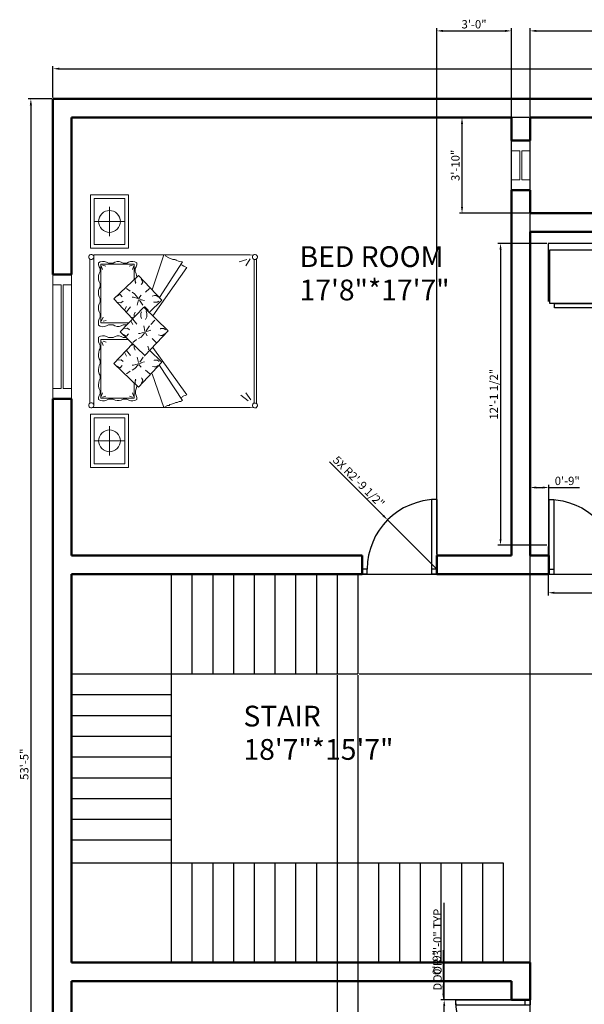
# Model space of a CAD drawing. Units: inches. Extents: x 2201 to 2875, y 1361 to 2074.
# Tile 2 of 4: x 2201 to 2474, y 1600 to 2074. Entities that reach past the tile are written whole.
import ezdxf

# ---------------------------------------------------------------- set-up
doc = ezdxf.new("R2010")
doc.units = ezdxf.units.IN
for name, color, linetype, lineweight in [('A-ANNO-DIMS', 2, 'Continuous', 18), ('A-AREA-IDEN', 7, 'Continuous', 25), ('A-FLOR-FIXT', 9, 'Continuous', 18), ('doors', 5, 'Continuous', 25), ('furniture', 8, 'Continuous', 18), ('stairs', 1, 'Continuous', 25), ('ventilator', 3, 'Continuous', 18), ('walls', 6, 'Continuous', 50), ('windows', 4, 'Continuous', 18)]:
    doc.layers.add(name, color=color, linetype=linetype, lineweight=lineweight)
doc.layers.add('TEFRIŞ', color=11, linetype='Continuous')
doc.styles.get("Standard").update_dxf_attribs({"font": 'arial.ttf'})
doc.dimstyles.new('ISO-25', dxfattribs={"dimtxt": 4, "dimasz": 3, "dimexe": 1.25, "dimexo": 0.625, "dimtad": 1, "dimlunit": 3, "dimtxsty": 'Standard', "dimcen": 2.5, "dimadec": 0, "dimazin": 0, "dimtfac": 1, "dimtmove": 0, "dimatfit": 3, "dimfxl": 1, "dimarcsym": 0})

# ---------------------------------------------------------------- blocks, each defined once
blk = doc.blocks.new('d-bed-3')
at = {"color": 0, "linetype": 'ByBlock'}
for p, q in [((0, 0), (0, -0.5)), ((0.7, 0), (0, 0)), ((0.7, -0.5), (0.7, 0)), ((0.782, -0.005), (0.786, 0.008)), ((0.782, -0.005), (0.786, 0.008)), ((0.786, 0.008), (0.797, 0.017)), ((0.786, 0.008), (0.797, 0.017)), ((0.797, 0.017), (0.808, 0.021)), ((0.797, 0.017), (0.808, 0.021)), ((0.808, 0.021), (0.821, 0.021)), ((0.808, 0.021), (0.821, 0.021)), ((0.821, 0.021), (0.835, 0.014)), ((0.821, 0.021), (0.835, 0.014)), ((0.835, 0.014), (0.841, 0.008)), ((0.835, 0.014), (0.843, 0.006)), ((0.839, 0.008), (2.73, 0.008)), ((0.841, 0.008), (2.73, 0.008)), ((0.843, 0.006), (0.848, -0.008)), ((2.723, -0.008), (2.728, 0.006)), ((2.728, 0.006), (2.736, 0.014)), ((2.73, 0.008), (2.736, 0.014)), ((2.736, 0.014), (2.751, 0.021)), ((2.736, 0.014), (2.751, 0.021)), ((2.751, 0.021), (2.764, 0.021)), ((2.751, 0.021), (2.764, 0.021)), ((2.764, 0.021), (2.775, 0.017)), ((2.764, 0.021), (2.775, 0.017)), ((2.775, 0.017), (2.786, 0.008)), ((2.775, 0.017), (2.786, 0.008)), ((2.786, 0.008), (2.79, -0.005)), ((2.786, 0.008), (2.79, -0.005)), ((2.871, -0.5), (2.871, 0)), ((2.871, 0), (3.571, 0)), ((3.571, 0), (3.571, -0.5)), ((0.05, -0.05), (0.05, -0.45)), ((0.65, -0.05), (0.05, -0.05)), ((0.35, -0.058), (0.35, -0.442)), ((0.65, -0.45), (0.65, -0.05)), ((0.782, -0.019), (0.782, -0.005)), ((0.782, -0.019), (0.782, -0.005)), ((0.786, -0.03), (0.782, -0.019)), ((0.786, -0.03), (0.782, -0.019)), ((0.786, -2.094), (0.786, -0.03)), ((0.795, -0.041), (0.786, -0.03)), ((0.786, -0.032), (0.786, -2.094)), ((0.806, -0.045), (0.795, -0.041)), ((0.819, -0.045), (0.806, -0.045)), ((0.832, -0.041), (0.819, -0.045)), ((2.753, -0.045), (0.819, -0.045)), ((0.841, -0.032), (0.832, -0.041)), ((0.848, -0.021), (0.841, -0.032)), ((0.848, -0.008), (0.848, -0.021)), ((0.878, -0.132), (0.891, -0.106)), ((0.891, -0.106), (0.918, -0.108)), ((0.918, -0.108), (0.944, -0.115)), ((0.944, -0.115), (0.968, -0.128)), ((0.968, -0.128), (1.006, -0.128)), ((1.006, -0.128), (1.032, -0.117)), ((1.032, -0.117), (1.059, -0.108)), ((1.059, -0.108), (1.085, -0.106)), ((1.085, -0.106), (1.113, -0.11)), ((1.113, -0.11), (1.14, -0.117)), ((1.14, -0.117), (1.166, -0.128)), ((1.166, -0.128), (1.203, -0.128)), ((1.203, -0.128), (1.229, -0.117)), ((1.229, -0.117), (1.257, -0.108)), ((1.257, -0.108), (1.283, -0.106)), ((1.283, -0.106), (1.311, -0.11)), ((1.311, -0.11), (1.338, -0.117)), ((1.338, -0.117), (1.362, -0.128)), ((1.362, -0.128), (1.401, -0.128)), ((1.401, -0.128), (1.425, -0.117)), ((1.425, -0.117), (1.451, -0.108)), ((1.451, -0.108), (1.48, -0.106)), ((1.48, -0.106), (1.509, -0.11)), ((1.509, -0.11), (1.536, -0.117)), ((1.536, -0.117), (1.56, -0.128)), ((1.56, -0.128), (1.599, -0.128)), ((1.599, -0.128), (1.623, -0.115)), ((1.623, -0.115), (1.647, -0.108)), ((1.647, -0.108), (1.676, -0.106)), ((1.676, -0.106), (1.708, -0.106)), ((1.708, -0.106), (1.719, -0.132)), ((1.849, -0.13), (1.863, -0.106)), ((1.863, -0.106), (1.895, -0.106)), ((1.895, -0.106), (1.922, -0.106)), ((1.922, -0.106), (1.948, -0.115)), ((1.948, -0.115), (1.972, -0.128)), ((1.972, -0.128), (2.01, -0.128)), ((2.01, -0.128), (2.036, -0.115)), ((2.036, -0.115), (2.063, -0.108)), ((2.063, -0.108), (2.091, -0.106)), ((2.091, -0.106), (2.117, -0.108)), ((2.117, -0.108), (2.144, -0.115)), ((2.144, -0.115), (2.17, -0.128)), ((2.17, -0.128), (2.207, -0.128)), ((2.207, -0.128), (2.233, -0.115)), ((2.233, -0.115), (2.261, -0.108)), ((2.261, -0.108), (2.287, -0.106)), ((2.287, -0.106), (2.315, -0.108)), ((2.315, -0.108), (2.342, -0.115)), ((2.342, -0.115), (2.366, -0.128)), ((2.366, -0.128), (2.405, -0.128)), ((2.405, -0.128), (2.429, -0.115)), ((2.429, -0.115), (2.455, -0.108)), ((2.455, -0.108), (2.484, -0.106)), ((2.484, -0.106), (2.513, -0.108)), ((2.513, -0.108), (2.54, -0.115)), ((2.54, -0.115), (2.564, -0.128)), ((2.564, -0.128), (2.603, -0.128)), ((2.603, -0.128), (2.627, -0.115)), ((2.627, -0.115), (2.651, -0.106)), ((2.651, -0.106), (2.68, -0.106)), ((2.68, -0.106), (2.691, -0.13)), ((2.723, -0.021), (2.723, -0.008)), ((2.73, -0.032), (2.723, -0.021)), ((2.739, -0.041), (2.73, -0.032)), ((2.753, -0.045), (2.739, -0.041)), ((2.766, -0.045), (2.753, -0.045)), ((2.777, -0.041), (2.766, -0.045)), ((2.777, -0.041), (2.766, -0.045)), ((2.766, -0.045), (2.786, -0.045)), ((2.786, -0.045), (2.766, -0.045)), ((2.786, -0.03), (2.777, -0.041)), ((2.786, -0.03), (2.777, -0.041)), ((2.79, -0.019), (2.786, -0.03)), ((2.79, -0.019), (2.786, -0.03)), ((2.786, -2.094), (2.786, -0.045)), ((2.79, -0.005), (2.79, -0.019)), ((2.79, -0.005), (2.79, -0.019)), ((2.921, -0.45), (2.921, -0.05)), ((2.921, -0.05), (3.521, -0.05)), ((3.221, -0.058), (3.221, -0.442)), ((3.521, -0.05), (3.521, -0.45)), ((0.158, -0.25), (0.542, -0.25)), ((0.872, -0.159), (0.878, -0.132)), ((0.874, -0.187), (0.872, -0.159)), ((0.883, -0.213), (0.874, -0.187)), ((0.896, -0.237), (0.883, -0.213)), ((0.896, -0.299), (0.896, -0.237)), ((0.907, -0.575), (0.907, -0.139)), ((0.907, -0.139), (1.676, -0.139)), ((0.922, -0.161), (0.933, -0.204)), ((0.929, -0.143), (0.977, -0.161)), ((1.647, -0.15), (1.599, -0.166)), ((1.654, -0.166), (1.643, -0.209)), ((1.676, -0.139), (1.676, -0.494)), ((1.717, -0.213), (1.702, -0.237)), ((1.702, -0.237), (1.702, -0.299)), ((1.726, -0.187), (1.717, -0.213)), ((1.719, -0.132), (1.726, -0.159)), ((1.726, -0.159), (1.726, -0.187)), ((1.843, -0.159), (1.849, -0.13)), ((1.845, -0.187), (1.843, -0.159)), ((1.854, -0.213), (1.845, -0.187)), ((1.867, -0.237), (1.854, -0.213)), ((1.867, -0.297), (1.867, -0.237)), ((2.662, -0.137), (1.893, -0.137)), ((1.893, -0.137), (1.893, -0.505)), ((1.915, -0.166), (1.926, -0.209)), ((1.922, -0.148), (1.97, -0.166)), ((2.64, -0.143), (2.592, -0.159)), ((2.647, -0.159), (2.636, -0.202)), ((2.662, -0.575), (2.662, -0.137)), ((2.688, -0.213), (2.673, -0.237)), ((2.673, -0.237), (2.673, -0.297)), ((2.697, -0.187), (2.688, -0.213)), ((2.691, -0.13), (2.697, -0.159)), ((2.697, -0.159), (2.697, -0.187)), ((3.414, -0.25), (3.029, -0.25)), ((0.876, -0.349), (0.883, -0.324)), ((0.876, -0.378), (0.876, -0.349)), ((0.883, -0.404), (0.876, -0.378)), ((0.883, -0.324), (0.896, -0.299)), ((1.054, -0.629), (1.362, -0.308)), ((1.329, -0.351), (1.307, -0.391)), ((1.362, -0.308), (1.619, -0.553)), ((1.405, -0.347), (1.412, -0.402)), ((1.702, -0.299), (1.717, -0.324)), ((1.717, -0.324), (1.724, -0.349)), ((1.724, -0.378), (1.717, -0.404)), ((1.724, -0.349), (1.724, -0.378)), ((1.847, -0.349), (1.854, -0.321)), ((1.847, -0.375), (1.847, -0.349)), ((1.854, -0.404), (1.847, -0.375)), ((1.854, -0.321), (1.867, -0.297)), ((2.207, -0.308), (1.948, -0.553)), ((2.163, -0.344), (2.157, -0.4)), ((2.515, -0.629), (2.207, -0.308)), ((2.241, -0.351), (2.263, -0.389)), ((2.673, -0.297), (2.688, -0.321)), ((2.688, -0.321), (2.695, -0.349)), ((2.695, -0.375), (2.688, -0.404)), ((2.695, -0.349), (2.695, -0.375)), ((0, -0.5), (0.7, -0.5)), ((0.05, -0.45), (0.65, -0.45)), ((0.874, -0.529), (0.883, -0.502)), ((0.896, -0.428), (0.883, -0.404)), ((0.883, -0.502), (0.896, -0.478)), ((0.896, -0.478), (0.896, -0.428)), ((0.922, -0.553), (0.933, -0.511)), ((1.225, -0.472), (1.263, -0.522)), ((1.307, -0.391), (1.335, -0.417)), ((1.412, -0.402), (1.39, -0.428)), ((1.501, -0.451), (1.46, -0.472)), ((1.467, -0.713), (1.775, -0.391)), ((1.533, -0.472), (1.467, -0.527)), ((1.717, -0.404), (1.702, -0.428)), ((1.702, -0.428), (1.702, -0.465)), ((1.742, -0.435), (1.719, -0.474)), ((1.719, -0.474), (1.749, -0.5)), ((1.775, -0.391), (2.098, -0.698)), ((1.823, -0.485), (1.801, -0.511)), ((1.819, -0.431), (1.823, -0.485)), ((1.867, -0.428), (1.854, -0.404)), ((1.867, -0.478), (1.867, -0.428)), ((2.036, -0.472), (2.102, -0.527)), ((2.069, -0.451), (2.109, -0.472)), ((2.157, -0.4), (2.179, -0.428)), ((2.263, -0.389), (2.233, -0.417)), ((2.344, -0.472), (2.307, -0.52)), ((2.647, -0.553), (2.636, -0.509)), ((2.688, -0.404), (2.673, -0.428)), ((2.673, -0.428), (2.673, -0.476)), ((2.673, -0.476), (2.688, -0.5)), ((2.688, -0.5), (2.697, -0.527)), ((3.571, -0.5), (2.871, -0.5)), ((3.521, -0.45), (2.921, -0.45)), ((0.872, -0.558), (0.874, -0.529)), ((0.878, -0.584), (0.872, -0.558)), ((0.891, -0.61), (0.878, -0.584)), ((0.918, -0.607), (0.891, -0.61)), ((1.109, -0.575), (0.907, -0.575)), ((0.944, -0.601), (0.918, -0.607)), ((0.929, -0.571), (0.977, -0.553)), ((0.968, -0.589), (0.944, -0.601)), ((1.006, -0.589), (0.968, -0.589)), ((1.032, -0.6), (1.006, -0.589)), ((1.059, -0.607), (1.032, -0.6)), ((1.379, -0.936), (1.054, -0.629)), ((1.076, -0.61), (1.059, -0.607)), ((1.105, -0.586), (1.127, -0.586)), ((1.127, -0.586), (1.148, -0.597)), ((1.148, -0.597), (1.131, -0.586)), ((1.131, -0.586), (1.159, -0.593)), ((1.296, -0.582), (1.274, -0.549)), ((1.346, -0.625), (1.296, -0.582)), ((1.314, -0.663), (1.351, -0.636)), ((1.34, -0.564), (1.34, -0.549)), ((1.357, -0.625), (1.34, -0.564)), ((1.368, -0.663), (1.357, -0.625)), ((1.373, -0.629), (1.445, -0.614)), ((1.566, -0.575), (1.538, -0.586)), ((1.597, -0.575), (1.566, -0.575)), ((1.599, -0.549), (1.614, -0.555)), ((1.638, -0.555), (1.676, -0.605)), ((1.708, -0.665), (1.687, -0.632)), ((1.753, -0.649), (1.753, -0.632)), ((1.911, -0.533), (1.874, -0.555)), ((1.944, -0.555), (1.878, -0.61)), ((1.97, -0.547), (1.95, -0.555)), ((1.968, -0.575), (2.004, -0.575)), ((2.004, -0.575), (2.032, -0.586)), ((2.039, -0.643), (2.043, -0.64)), ((2.196, -0.629), (2.124, -0.612)), ((2.19, -0.936), (2.515, -0.629)), ((2.201, -0.663), (2.212, -0.623)), ((2.212, -0.623), (2.229, -0.564)), ((2.256, -0.663), (2.218, -0.634)), ((2.222, -0.623), (2.274, -0.58)), ((2.229, -0.564), (2.229, -0.547)), ((2.274, -0.58), (2.296, -0.547)), ((2.438, -0.586), (2.409, -0.591)), ((2.442, -0.586), (2.42, -0.597)), ((2.42, -0.597), (2.438, -0.586)), ((2.464, -0.586), (2.442, -0.586)), ((2.46, -0.575), (2.662, -0.575)), ((2.513, -0.605), (2.496, -0.607)), ((2.54, -0.6), (2.513, -0.605)), ((2.564, -0.586), (2.54, -0.6)), ((2.603, -0.586), (2.564, -0.586)), ((2.64, -0.569), (2.592, -0.553)), ((2.627, -0.6), (2.603, -0.586)), ((2.651, -0.607), (2.627, -0.6)), ((2.68, -0.607), (2.651, -0.607)), ((2.691, -0.584), (2.68, -0.607)), ((2.697, -0.555), (2.691, -0.584)), ((2.697, -0.527), (2.697, -0.555)), ((1.105, -0.669), (1.142, -0.685)), ((1.142, -0.685), (1.164, -0.674)), ((1.164, -0.674), (1.175, -0.669)), ((1.225, -0.779), (1.274, -0.724)), ((1.373, -0.669), (1.384, -0.707)), ((1.379, -0.647), (1.445, -0.691)), ((1.467, -0.713), (1.46, -0.707)), ((1.79, -1.019), (1.467, -0.713)), ((1.555, -0.767), (1.54, -0.763)), ((1.555, -0.767), (1.577, -0.756)), ((1.577, -0.756), (1.588, -0.752)), ((1.76, -0.709), (1.708, -0.665)), ((1.726, -0.745), (1.764, -0.72)), ((1.771, -0.709), (1.753, -0.649)), ((1.782, -0.745), (1.771, -0.709)), ((1.786, -0.713), (1.856, -0.698)), ((1.786, -0.752), (1.797, -0.79)), ((2.098, -0.698), (1.79, -1.019)), ((1.79, -0.731), (1.856, -0.774)), ((1.972, -0.741), (1.939, -0.724)), ((1.976, -0.66), (1.95, -0.671)), ((2.01, -0.741), (1.972, -0.741)), ((2.017, -0.66), (1.976, -0.66)), ((2.05, -0.731), (2.01, -0.741)), ((2.039, -0.671), (2.017, -0.66)), ((2.19, -0.936), (2.028, -0.77)), ((2.054, -0.761), (2.109, -0.707)), ((2.19, -0.645), (2.124, -0.689)), ((2.196, -0.667), (2.185, -0.707)), ((2.344, -0.776), (2.296, -0.722)), ((2.405, -0.674), (2.394, -0.667)), ((2.427, -0.685), (2.405, -0.674)), ((2.464, -0.667), (2.427, -0.685)), ((0.786, -0.961), (1.229, -0.807)), ((0.95, -1.261), (1.571, -0.818)), ((1.318, -0.838), (1.324, -0.812)), ((1.318, -0.86), (1.318, -0.838)), ((1.335, -0.888), (1.318, -0.86)), ((1.379, -0.936), (1.536, -0.776)), ((1.39, -0.899), (1.405, -0.877)), ((1.405, -0.834), (1.401, -0.834)), ((1.405, -0.877), (1.405, -0.834)), ((1.638, -0.862), (1.687, -0.807)), ((1.73, -0.921), (1.738, -0.894)), ((1.928, -0.845), (1.874, -0.79)), ((2.618, -1.261), (1.985, -0.816)), ((2.163, -0.876), (2.163, -0.832)), ((2.163, -0.832), (2.168, -0.832)), ((2.179, -0.897), (2.163, -0.876)), ((2.233, -0.886), (2.252, -0.86)), ((2.252, -0.838), (2.245, -0.809)), ((2.252, -0.86), (2.252, -0.838)), ((2.783, -0.961), (2.328, -0.807)), ((0.813, -1.012), (0.786, -0.961)), ((0.813, -1.033), (0.813, -1.012)), ((0.878, -1.206), (1.335, -0.906)), ((1.73, -0.943), (1.73, -0.921)), ((1.749, -0.972), (1.73, -0.943)), ((1.801, -0.983), (1.819, -0.961)), ((1.819, -0.917), (1.812, -0.917)), ((1.819, -0.961), (1.819, -0.917)), ((2.691, -1.206), (2.225, -0.906)), ((2.746, -1.026), (2.723, -1.081)), ((2.768, -0.989), (2.746, -1.026)), ((2.779, -0.983), (2.768, -0.989)), ((2.783, -0.961), (2.779, -0.983)), ((0.824, -1.041), (0.813, -1.033)), ((0.83, -1.063), (0.824, -1.041)), ((0.835, -1.075), (0.83, -1.063)), ((0.845, -1.103), (0.835, -1.075)), ((0.852, -1.119), (0.845, -1.103)), ((0.852, -1.136), (0.852, -1.119)), ((0.863, -1.162), (0.852, -1.136)), ((2.712, -1.125), (2.695, -1.162)), ((2.717, -1.119), (2.712, -1.125)), ((2.723, -1.108), (2.717, -1.119)), ((2.723, -1.081), (2.723, -1.108)), ((0.867, -1.19), (0.863, -1.162)), ((0.874, -1.195), (0.867, -1.19)), ((0.878, -1.206), (0.874, -1.195)), ((0.922, -1.202), (0.911, -1.184)), ((0.929, -1.206), (0.922, -1.202)), ((0.94, -1.224), (0.929, -1.206)), ((0.944, -1.239), (0.94, -1.224)), ((0.95, -1.261), (0.944, -1.239)), ((2.625, -1.239), (2.618, -1.261)), ((2.636, -1.224), (2.625, -1.239)), ((2.647, -1.202), (2.636, -1.224)), ((2.658, -1.184), (2.647, -1.202)), ((2.695, -1.162), (2.691, -1.206)), ((0.874, -2.067), (0.946, -1.969)), ((0.885, -2.1), (0.979, -2.034)), ((2.73, -2.094), (2.642, -2.034)), ((2.723, -2.05), (2.691, -1.947)), ((0.78, -2.148), (0.786, -2.135)), ((0.78, -2.148), (0.786, -2.135)), ((0.78, -2.159), (0.78, -2.148)), ((0.78, -2.148), (0.78, -2.159)), ((0.784, -2.172), (0.78, -2.159)), ((0.784, -2.172), (0.78, -2.159)), ((0.793, -2.181), (0.784, -2.172)), ((0.793, -2.181), (0.784, -2.172)), ((0.789, -2.132), (0.786, -2.094)), ((0.786, -2.094), (0.789, -2.13)), ((0.786, -2.135), (0.795, -2.126)), ((0.786, -2.135), (0.789, -2.132)), ((0.806, -2.188), (0.793, -2.181)), ((0.806, -2.188), (0.793, -2.181)), ((0.795, -2.126), (0.808, -2.121)), ((0.817, -2.188), (0.806, -2.188)), ((0.817, -2.188), (0.806, -2.188)), ((0.808, -2.121), (0.819, -2.121)), ((0.83, -2.183), (0.817, -2.188)), ((0.83, -2.183), (0.817, -2.188)), ((0.819, -2.121), (0.832, -2.128)), ((0.839, -2.174), (0.83, -2.183)), ((0.837, -2.177), (0.83, -2.183)), ((0.832, -2.128), (0.841, -2.137)), ((2.733, -2.177), (0.837, -2.177)), ((0.845, -2.161), (0.839, -2.174)), ((0.839, -2.177), (2.73, -2.177)), ((0.841, -2.137), (0.845, -2.15)), ((2.726, -2.144), (0.845, -2.144)), ((0.845, -2.15), (0.845, -2.161)), ((2.728, -2.137), (2.723, -2.15)), ((2.723, -2.15), (2.723, -2.161)), ((2.723, -2.161), (2.73, -2.174)), ((2.736, -2.128), (2.728, -2.137)), ((2.73, -2.174), (2.739, -2.183)), ((2.739, -2.183), (2.733, -2.177)), ((2.751, -2.121), (2.736, -2.128)), ((2.753, -2.188), (2.739, -2.183)), ((2.739, -2.183), (2.753, -2.188)), ((2.762, -2.121), (2.751, -2.121)), ((2.764, -2.188), (2.753, -2.188)), ((2.753, -2.188), (2.764, -2.188)), ((2.775, -2.126), (2.762, -2.121)), ((2.777, -2.181), (2.764, -2.188)), ((2.764, -2.188), (2.777, -2.181)), ((2.783, -2.135), (2.775, -2.126)), ((2.786, -2.172), (2.777, -2.181)), ((2.777, -2.181), (2.786, -2.172)), ((2.786, -2.094), (2.778, -2.13)), ((2.778, -2.13), (2.783, -2.135)), ((2.779, -2.128), (2.786, -2.094)), ((2.783, -2.135), (2.79, -2.148)), ((2.79, -2.148), (2.783, -2.135)), ((2.79, -2.159), (2.786, -2.172)), ((2.786, -2.172), (2.79, -2.159)), ((2.79, -2.148), (2.79, -2.159)), ((2.79, -2.159), (2.79, -2.148))]:
    blk.add_line(p, q, dxfattribs=at)
blk.add_ellipse((0.35, -0.25), major_axis=(-0.101, 0.101), ratio=1, dxfattribs=at)
at = {"color": 0, "linetype": 'ByBlock', "extrusion": (0, 0, -1)}
blk.add_ellipse((3.221, -0.25), major_axis=(0.101, 0.101), ratio=1, dxfattribs=at)
blk = doc.blocks.new('A$C008029BD')
at = {"layer": 'TEFRIŞ', "ltscale": 0.05}
for p, q in [((0, 0), (0, -3.55)), ((3.37, 0), (0, 0)), ((3.37, 0), (3.37, -0.6)), ((1.522, -0.4), (0, -0.4)), ((3.37, -0.4), (2.083, -0.4)), ((0.05, -0.581), (0.05, -1.869)), ((0.05, -0.581), (0.55, -0.581)), ((0.096, -0.617), (0.454, -0.617)), ((0.099, -0.659), (0.457, -0.659)), ((0.55, -0.581), (0.55, -1.869)), ((0.6, -2.71), (0.6, -0.6)), ((3.37, -0.6), (0.6, -0.6)), ((0.086, -1.773), (0.086, -0.677)), ((0.113, -0.954), (0.113, -0.695)), ((0.493, -0.695), (0.493, -0.954)), ((0.514, -0.677), (0.514, -1.773)), ((0.23, -0.846), (0.229, -0.967)), ((0.28, -0.846), (0.277, -1.158)), ((0.096, -1.024), (0.454, -1.024)), ((0.457, -0.99), (0.099, -0.99)), ((0.11, -1.319), (0.11, -1.06)), ((0.228, -1.02), (0.227, -1.159)), ((0.49, -1.06), (0.49, -1.319)), ((0.454, -1.355), (0.096, -1.355)), ((0.096, -1.391), (0.454, -1.391)), ((0.11, -1.773), (0.11, -1.427)), ((0.154, -1.773), (0.154, -1.427)), ((0.214, -1.773), (0.214, -1.427)), ((0.274, -1.773), (0.274, -1.427)), ((0.334, -1.773), (0.334, -1.427)), ((0.39, -1.773), (0.39, -1.427)), ((0.444, -1.773), (0.444, -1.427)), ((0.49, -1.427), (0.49, -1.773)), ((0.55, -1.869), (0.05, -1.869)), ((0.454, -1.809), (0.096, -1.809)), ((0.454, -1.833), (0.096, -1.833)), ((0, -2.025), (0.4, -2.025)), ((0.4, -2.71), (0.4, -2.025)), ((0, -2.71), (0.6, -2.71)), ((0, -3.55), (0.65, -3.55))]:
    blk.add_line(p, q, dxfattribs=at)
at = {"layer": 'TEFRIŞ'}
blk.add_line((1.969, -0.05), (1.969, -0.572), dxfattribs=at)
at = {"layer": 'TEFRIŞ', "ltscale": 0.05}
for points in [[(1.522, -0.05), (2.083, -0.05), (2.083, -0.572), (1.522, -0.572)], [(0.67, -2.73), (0.67, -3.53), (0.07, -3.53), (0.07, -2.73)], [(0.72, -2.78), (0.72, -3.48), (0.67, -3.48), (0.67, -2.78)]]:
    blk.add_lwpolyline(points, close=True, dxfattribs=at)
at = {"layer": 'TEFRIŞ', "const_width": 0.025}
for points in [[(2.014, -0.123, 1), (2.039, -0.123, 1)], [(2.014, -0.236, 1), (2.039, -0.236, 1)], [(2.014, -0.327, 1), (2.039, -0.327, 1)], [(2.014, -0.44, 1), (2.039, -0.44, 1)]]:
    blk.add_lwpolyline(points, format="xyb", close=True, dxfattribs=at)
at = {"layer": 'TEFRIŞ', "ltscale": 0.05}
for centre, radius in [((1.628, -0.164), 0.0505), ((1.628, -0.45), 0.0505), ((0.255, -0.82), 0.036), ((0.252, -1.184), 0.036)]:
    blk.add_circle(centre, radius, dxfattribs=at)
at = {"layer": 'TEFRIŞ'}
for centre in [(1.88, -0.164), (1.88, -0.45)]:
    blk.add_circle(centre, 0.0505, dxfattribs=at)
at = {"layer": 'TEFRIŞ', "ltscale": 0.05}
for centre, radius, start, end in [((0.108, -0.649), 0.0351, 110.4976, 230.5777), ((0.118, -0.673), 0.023, 143.9853, 258.5157), ((0.454, -0.677), 0.06, 0, 90), ((0.457, -0.695), 0.036, 0, 90), ((0.118, -0.976), 0.023, 101.4843, 216.0147), ((0.457, -0.954), 0.036, 270, 0), ((0.115, -1.038), 0.023, 143.9853, 258.5157), ((0.454, -1.06), 0.036, 0, 90), ((0.115, -1.341), 0.023, 101.4843, 216.0147), ((0.454, -1.319), 0.036, 270, 0), ((0.115, -1.405), 0.023, 143.9853, 258.5157), ((0.454, -1.427), 0.036, 0, 90), ((0.108, -1.801), 0.0351, 129.4223, 249.5024), ((0.115, -1.796), 0.023, 101.4843, 216.0147), ((0.454, -1.773), 0.06, 270, 0), ((0.454, -1.773), 0.036, 270, 0)]:
    blk.add_arc(centre, radius, start, end, dxfattribs=at)
blk = doc.blocks.new('*D9')
at = {"layer": 'A-ANNO-DIMS', "color": 0, "lineweight": -2, "transparency": 16777216}
for p, q in [((2217.4, 2036.51), (2217.4, 2051.71)), ((2220.4, 2050.46), (2836.4, 2050.46)), ((2839.4, 2036.51), (2839.4, 2051.71))]:
    blk.add_line(p, q, dxfattribs=at)
at = {"layer": 'A-ANNO-DIMS', "color": 0, "transparency": 16777216}
for points in [[(2220.4, 2050.96), (2220.4, 2049.96), (2217.4, 2050.46)], [(2836.4, 2050.96), (2836.4, 2049.96), (2839.4, 2050.46)]]:
    blk.add_solid(points, dxfattribs=at)
at = {"layer": 'Defpoints', "color": 0, "transparency": 16777216}
for p in [(2839.4, 2050.46), (2217.4, 2035.88), (2839.4, 2035.88)]:
    blk.add_point(p, dxfattribs=at)
at = {"layer": 'A-ANNO-DIMS', "color": 0, "transparency": 16777216, "insert": (2528.4, 2053.13), "char_height": 4, "attachment_point": 5}
blk.add_mtext('51\'-10"', dxfattribs=at)
blk = doc.blocks.new('*D11')
at = {"layer": 'A-ANNO-DIMS', "color": 0, "lineweight": -2, "transparency": 16777216}
for p, q in [((2216.78, 2035.88), (2205.5, 2035.88)), ((2206.75, 2032.88), (2206.75, 1397.88)), ((2216.78, 1394.88), (2205.5, 1394.88))]:
    blk.add_line(p, q, dxfattribs=at)
at = {"layer": 'A-ANNO-DIMS', "color": 0, "transparency": 16777216}
for points in [[(2206.25, 2032.88), (2207.25, 2032.88), (2206.75, 2035.88)], [(2206.25, 1397.88), (2207.25, 1397.88), (2206.75, 1394.88)]]:
    blk.add_solid(points, dxfattribs=at)
at = {"layer": 'Defpoints', "color": 0, "transparency": 16777216}
for p in [(2217.4, 2035.88), (2206.75, 1394.88), (2217.4, 1394.88)]:
    blk.add_point(p, dxfattribs=at)
at = {"layer": 'A-ANNO-DIMS', "color": 0, "transparency": 16777216, "insert": (2204.09, 1715.38), "char_height": 4, "attachment_point": 5, "rotation": 90}
blk.add_mtext('53\'-5"', dxfattribs=at)
blk = doc.blocks.new('DOOR-SWING-36IN')
for p, q in [((33.5, 36), (33.5, 0)), ((36, 36), (33.5, 36)), ((36, 36), (36, 0)), ((2.5, 2.5), (0, 2.5)), ((0, 0), (0, 2.5)), ((2.5, 0), (2.5, 2.5)), ((36, 2.5), (33.5, 2.5)), ((2.5, 0), (0, 0)), ((36, 0), (33.5, 0))]:
    blk.add_line(p, q)
blk.add_arc((36, 2.5), 33.5, 90, 180)
blk = doc.blocks.new('WIN-60IN')
for p, q in [((0, 9), (60, 9)), ((0, 0), (0, 9)), ((5, 5), (5, 9)), ((55, 5), (5, 5)), ((55, 9), (55, 5)), ((60, 9), (60, 0)), ((5, 0), (5, 4)), ((55, 4), (5, 4)), ((55, 4), (55, 0)), ((60, 0), (0, 0))]:
    blk.add_line(p, q)
blk = doc.blocks.new('VENT-24IN')
for p, q in [((0, 24), (0, 0)), ((9, 24), (0, 24)), ((9, 0), (9, 24)), ((4, 19), (0, 19)), ((4, 19), (4, 5)), ((9, 19), (5, 19)), ((5, 19), (5, 5)), ((0, 5), (4, 5)), ((5, 5), (9, 5)), ((0, 0), (9, 0))]:
    blk.add_line(p, q)
blk = doc.blocks.new('*D18')
at = {"layer": 'A-ANNO-DIMS', "color": 0, "lineweight": -2, "transparency": 16777216}
for p, q in [((2406, 1601.88), (2406, 1648.63)), ((2410.78, 1601.88), (2404.75, 1601.88)), ((2406, 1568.88), (2406, 1598.88)), ((2410.78, 1565.88), (2404.75, 1565.88))]:
    blk.add_line(p, q, dxfattribs=at)
at = {"layer": 'A-ANNO-DIMS', "color": 0, "transparency": 16777216}
for points in [[(2405.5, 1598.88), (2406.5, 1598.88), (2406, 1601.88)], [(2405.5, 1568.88), (2406.5, 1568.88), (2406, 1565.88)]]:
    blk.add_solid(points, dxfattribs=at)
at = {"layer": 'Defpoints', "color": 0, "transparency": 16777216}
for p in [(2406, 1601.88), (2411.4, 1601.88), (2411.4, 1565.88)]:
    blk.add_point(p, dxfattribs=at)
at = {"layer": 'A-ANNO-DIMS', "color": 0, "transparency": 16777216, "insert": (2403.31, 1626.76), "char_height": 4, "attachment_point": 5, "rotation": 90}
blk.add_mtext('DOOR 3\'-0" TYP.', dxfattribs=at)
blk = doc.blocks.new('*D34')
at = {"layer": 'A-ANNO-DIMS', "color": 0, "lineweight": -2, "transparency": 16777216}
for p, q in [((2456.14, 1820.31), (2456.14, 1796.72)), ((2609.26, 1820.31), (2609.26, 1796.72)), ((2459.14, 1797.97), (2606.26, 1797.97))]:
    blk.add_line(p, q, dxfattribs=at)
at = {"layer": 'A-ANNO-DIMS', "color": 0, "transparency": 16777216}
for points in [[(2459.14, 1798.47), (2459.14, 1797.47), (2456.14, 1797.97)], [(2606.26, 1798.47), (2606.26, 1797.47), (2609.26, 1797.97)]]:
    blk.add_solid(points, dxfattribs=at)
at = {"layer": 'Defpoints', "color": 0, "transparency": 16777216}
for p in [(2456.14, 1820.94), (2609.26, 1820.94), (2609.26, 1797.97)]:
    blk.add_point(p, dxfattribs=at)
at = {"layer": 'A-ANNO-DIMS', "color": 0, "transparency": 16777216, "insert": (2532.7, 1800.66), "char_height": 4, "attachment_point": 5}
blk.add_mtext('KITCHEN UNITS 12\'-9"', dxfattribs=at)
blk = doc.blocks.new('*D35')
at = {"layer": 'A-ANNO-DIMS', "color": 0, "lineweight": -2, "transparency": 16777216}
for p, q in [((2455.51, 1966.3), (2431.92, 1966.3)), ((2433.17, 1963.3), (2433.17, 1823.94)), ((2455.51, 1820.94), (2431.92, 1820.94))]:
    blk.add_line(p, q, dxfattribs=at)
at = {"layer": 'A-ANNO-DIMS', "color": 0, "transparency": 16777216}
for points in [[(2432.67, 1963.3), (2433.67, 1963.3), (2433.17, 1966.3)], [(2432.67, 1823.94), (2433.67, 1823.94), (2433.17, 1820.94)]]:
    blk.add_solid(points, dxfattribs=at)
at = {"layer": 'Defpoints', "color": 0, "transparency": 16777216}
for p in [(2456.14, 1966.3), (2433.17, 1820.94), (2456.14, 1820.94)]:
    blk.add_point(p, dxfattribs=at)
at = {"layer": 'A-ANNO-DIMS', "color": 0, "transparency": 16777216, "insert": (2430.47, 1893.62), "char_height": 4, "attachment_point": 5, "rotation": 90}
blk.add_mtext('12\'-1 1/2"', dxfattribs=at)
blk = doc.blocks.new('*D42')
at = {"layer": 'A-ANNO-DIMS', "color": 0, "lineweight": -2, "transparency": 16777216}
for p, q in [((2446.78, 2026.88), (2413.35, 2026.88)), ((2414.6, 1983.88), (2414.6, 2023.88)), ((2446.78, 1980.88), (2413.35, 1980.88))]:
    blk.add_line(p, q, dxfattribs=at)
at = {"layer": 'A-ANNO-DIMS', "color": 0, "transparency": 16777216}
for points in [[(2414.1, 2023.88), (2415.1, 2023.88), (2414.6, 2026.88)], [(2414.1, 1983.88), (2415.1, 1983.88), (2414.6, 1980.88)]]:
    blk.add_solid(points, dxfattribs=at)
at = {"layer": 'Defpoints', "color": 0, "transparency": 16777216}
for p in [(2414.6, 2026.88), (2447.4, 2026.88), (2447.4, 1980.88)]:
    blk.add_point(p, dxfattribs=at)
at = {"layer": 'A-ANNO-DIMS', "color": 0, "transparency": 16777216, "insert": (2411.93, 2003.88), "char_height": 4, "attachment_point": 5, "rotation": 90}
blk.add_mtext('3\'-10"', dxfattribs=at)
blk = doc.blocks.new('*D49')
at = {"layer": 'A-ANNO-DIMS', "color": 0, "lineweight": -2, "transparency": 16777216}
for p, q in [((2402.4, 1816.51), (2402.4, 2069.93)), ((2405.4, 2068.68), (2435.4, 2068.68)), ((2438.4, 1816.51), (2438.4, 2069.93))]:
    blk.add_line(p, q, dxfattribs=at)
at = {"layer": 'A-ANNO-DIMS', "color": 0, "transparency": 16777216}
for points in [[(2405.4, 2069.18), (2405.4, 2068.18), (2402.4, 2068.68)], [(2435.4, 2069.18), (2435.4, 2068.18), (2438.4, 2068.68)]]:
    blk.add_solid(points, dxfattribs=at)
at = {"layer": 'Defpoints', "color": 0, "transparency": 16777216}
for p in [(2438.4, 2068.68), (2402.4, 1815.88), (2438.4, 1815.88)]:
    blk.add_point(p, dxfattribs=at)
at = {"layer": 'A-ANNO-DIMS', "color": 0, "transparency": 16777216, "insert": (2420.4, 2071.35), "char_height": 4, "attachment_point": 5}
blk.add_mtext('3\'-0"', dxfattribs=at)
blk = doc.blocks.new('*D50')
at = {"layer": 'A-ANNO-DIMS', "color": 0, "lineweight": -2, "transparency": 16777216}
for p, q in [((2365.03, 1806.88), (2873.45, 1806.88)), ((2872.2, 1761.88), (2872.2, 1803.88)), ((2365.03, 1758.88), (2873.45, 1758.88))]:
    blk.add_line(p, q, dxfattribs=at)
at = {"layer": 'A-ANNO-DIMS', "color": 0, "transparency": 16777216}
for points in [[(2871.7, 1803.88), (2872.7, 1803.88), (2872.2, 1806.88)], [(2871.7, 1761.88), (2872.7, 1761.88), (2872.2, 1758.88)]]:
    blk.add_solid(points, dxfattribs=at)
at = {"layer": 'Defpoints', "color": 0, "transparency": 16777216}
for p in [(2364.4, 1806.88), (2872.2, 1806.88), (2364.4, 1758.88)]:
    blk.add_point(p, dxfattribs=at)
at = {"layer": 'A-ANNO-DIMS', "color": 0, "transparency": 16777216, "insert": (2869.54, 1782.88), "char_height": 4, "attachment_point": 5, "rotation": 90}
blk.add_mtext('4\'-0"', dxfattribs=at)
blk = doc.blocks.new('*D51')
at = {"layer": 'A-ANNO-DIMS', "color": 0, "lineweight": -2, "transparency": 16777216}
for p, q in [((2354.4, 1758.26), (2354.4, 1360.83)), ((2364.4, 1758.26), (2364.4, 1360.83)), ((2357.4, 1362.08), (2361.4, 1362.08)), ((2364.4, 1362.08), (2382.39, 1362.08))]:
    blk.add_line(p, q, dxfattribs=at)
at = {"layer": 'A-ANNO-DIMS', "color": 0, "transparency": 16777216}
for points in [[(2357.4, 1362.58), (2357.4, 1361.58), (2354.4, 1362.08)], [(2361.4, 1362.58), (2361.4, 1361.58), (2364.4, 1362.08)]]:
    blk.add_solid(points, dxfattribs=at)
at = {"layer": 'Defpoints', "color": 0, "transparency": 16777216}
for p in [(2354.4, 1758.88), (2364.4, 1758.88), (2364.4, 1362.08)]:
    blk.add_point(p, dxfattribs=at)
at = {"layer": 'A-ANNO-DIMS', "color": 0, "transparency": 16777216, "insert": (2374.9, 1364.75), "char_height": 4, "attachment_point": 5}
blk.add_mtext('0\'-10"', dxfattribs=at)
blk = doc.blocks.new('*D52')
at = {"layer": 'A-ANNO-DIMS', "color": 0, "lineweight": -2, "transparency": 16777216}
for p, q in [((2447.4, 1816.51), (2447.4, 1849.93)), ((2450.4, 1848.68), (2453.4, 1848.68)), ((2456.4, 1816.51), (2456.4, 1849.93)), ((2456.4, 1848.68), (2471.29, 1848.68))]:
    blk.add_line(p, q, dxfattribs=at)
at = {"layer": 'A-ANNO-DIMS', "color": 0, "transparency": 16777216}
for points in [[(2450.4, 1849.18), (2450.4, 1848.18), (2447.4, 1848.68)], [(2453.4, 1849.18), (2453.4, 1848.18), (2456.4, 1848.68)]]:
    blk.add_solid(points, dxfattribs=at)
at = {"layer": 'Defpoints', "color": 0, "transparency": 16777216}
for p in [(2456.4, 1848.68), (2447.4, 1815.88), (2456.4, 1815.88)]:
    blk.add_point(p, dxfattribs=at)
at = {"layer": 'A-ANNO-DIMS', "color": 0, "transparency": 16777216, "insert": (2465.34, 1851.35), "char_height": 4, "attachment_point": 5}
blk.add_mtext('0\'-9"', dxfattribs=at)
blk = doc.blocks.new('*D54')
at = {"layer": 'A-ANNO-DIMS', "color": 0, "lineweight": -2, "transparency": 16777216}
for p, q in [((2405.6, 1610.88), (2405.6, 1625.77)), ((2437.78, 1610.88), (2404.35, 1610.88)), ((2405.6, 1604.88), (2405.6, 1607.88)), ((2437.78, 1601.88), (2404.35, 1601.88))]:
    blk.add_line(p, q, dxfattribs=at)
at = {"layer": 'A-ANNO-DIMS', "color": 0, "transparency": 16777216}
for points in [[(2405.1, 1607.88), (2406.1, 1607.88), (2405.6, 1610.88)], [(2405.1, 1604.88), (2406.1, 1604.88), (2405.6, 1601.88)]]:
    blk.add_solid(points, dxfattribs=at)
at = {"layer": 'Defpoints', "color": 0, "transparency": 16777216}
for p in [(2405.6, 1610.88), (2438.4, 1610.88), (2438.4, 1601.88)]:
    blk.add_point(p, dxfattribs=at)
at = {"layer": 'A-ANNO-DIMS', "color": 0, "transparency": 16777216, "insert": (2402.94, 1619.82), "char_height": 4, "attachment_point": 5, "rotation": 90}
blk.add_mtext('0\'-9"', dxfattribs=at)
blk = doc.blocks.new('*D56')
at = {"layer": 'A-ANNO-DIMS', "color": 0, "lineweight": -2, "transparency": 16777216}
for p, q in [((2447.4, 1395.51), (2447.4, 2069.93)), ((2450.4, 2068.68), (2612.4, 2068.68)), ((2615.4, 1395.51), (2615.4, 2069.93))]:
    blk.add_line(p, q, dxfattribs=at)
at = {"layer": 'A-ANNO-DIMS', "color": 0, "transparency": 16777216}
for points in [[(2450.4, 2069.18), (2450.4, 2068.18), (2447.4, 2068.68)], [(2612.4, 2069.18), (2612.4, 2068.18), (2615.4, 2068.68)]]:
    blk.add_solid(points, dxfattribs=at)
at = {"layer": 'Defpoints', "color": 0, "transparency": 16777216}
for p in [(2615.4, 2068.68), (2447.4, 1394.88), (2615.4, 1394.88)]:
    blk.add_point(p, dxfattribs=at)
at = {"layer": 'A-ANNO-DIMS', "color": 0, "transparency": 16777216, "insert": (2531.4, 2071.35), "char_height": 4, "attachment_point": 5}
blk.add_mtext('14\'-0"', dxfattribs=at)
blk = doc.blocks.new('*D60')
at = {"layer": 'A-ANNO-DIMS', "color": 0, "lineweight": -2, "transparency": 16777216}
for p, q in [((2350.7, 1861.09), (2376.59, 1835.19)), ((2402.4, 1809.38), (2378.72, 1833.07))]:
    blk.add_line(p, q, dxfattribs=at)
at = {"layer": 'A-ANNO-DIMS', "color": 0, "transparency": 16777216}
blk.add_solid([(2376.95, 1835.55), (2376.24, 1834.84), (2378.72, 1833.07)], dxfattribs=at)
at = {"layer": 'Defpoints', "color": 0, "transparency": 16777216}
for p in [(2378.72, 1833.07), (2402.4, 1809.38)]:
    blk.add_point(p, dxfattribs=at)
at = {"layer": 'A-ANNO-DIMS', "color": 0, "transparency": 16777216, "insert": (2364.49, 1851.11), "char_height": 4, "attachment_point": 5, "rotation": 314.9991}
blk.add_mtext('5X R2\'-9 1/2"', dxfattribs=at)

msp = doc.modelspace()

# ---------------------------------------------------------------- linework, layer by layer
at = {"layer": 'stairs'}
for p, q in [((2366.403, 1806.883), (2226.403, 1806.883)), ((2226.403, 1806.883), (2226.403, 1619.883)), ((2274.403, 1806.883), (2274.403, 1619.883)), ((2284.403, 1806.883), (2284.403, 1758.883)), ((2294.403, 1806.883), (2294.403, 1758.883)), ((2304.403, 1806.883), (2304.403, 1758.883)), ((2314.403, 1806.883), (2314.403, 1758.883)), ((2324.403, 1806.883), (2324.403, 1758.883)), ((2334.403, 1806.883), (2334.403, 1758.883)), ((2344.403, 1806.883), (2344.403, 1758.883)), ((2354.403, 1806.883), (2354.403, 1758.883)), ((2364.403, 1806.883), (2364.403, 1758.883)), ((2226.403, 1758.883), (2364.403, 1758.883)), ((2226.403, 1748.883), (2274.403, 1748.883)), ((2226.403, 1738.883), (2274.403, 1738.883)), ((2226.403, 1728.883), (2274.403, 1728.883)), ((2226.403, 1718.883), (2274.403, 1718.883)), ((2226.403, 1708.883), (2274.403, 1708.883)), ((2226.403, 1698.883), (2274.403, 1698.883)), ((2226.403, 1688.883), (2274.403, 1688.883)), ((2226.403, 1678.883), (2274.403, 1678.883)), ((2226.403, 1667.883), (2434.403, 1667.883)), ((2284.403, 1667.883), (2284.403, 1619.883)), ((2294.403, 1667.883), (2294.403, 1619.883)), ((2304.403, 1667.883), (2304.403, 1619.883)), ((2314.403, 1667.883), (2314.403, 1619.883)), ((2324.403, 1667.883), (2324.403, 1619.883)), ((2334.403, 1667.883), (2334.403, 1619.883)), ((2344.403, 1667.883), (2344.403, 1619.883)), ((2354.403, 1667.883), (2354.403, 1619.883)), ((2364.403, 1667.883), (2364.403, 1619.883)), ((2374.403, 1667.883), (2374.403, 1619.883)), ((2384.403, 1667.883), (2384.403, 1619.883)), ((2394.403, 1667.883), (2394.403, 1619.883)), ((2404.403, 1667.883), (2404.403, 1619.883)), ((2414.403, 1667.883), (2414.403, 1619.883)), ((2424.403, 1667.883), (2424.403, 1619.883)), ((2434.403, 1667.883), (2434.403, 1619.883)), ((2226.403, 1619.883), (2434.403, 1619.883))]:
    msp.add_line(p, q, dxfattribs=at)
at = {"layer": 'walls'}
for p, q in [((2217.403, 2035.883), (2839.403, 2035.883)), ((2217.403, 2035.883), (2217.403, 1951.383)), ((2226.403, 2026.883), (2438.403, 2026.883)), ((2226.403, 2026.883), (2226.403, 1951.383)), ((2438.403, 2026.883), (2438.403, 2015.883)), ((2447.403, 2026.883), (2447.403, 2015.883)), ((2447.403, 2026.883), (2615.403, 2026.883)), ((2447.403, 2015.883), (2438.403, 2015.883)), ((2438.403, 1991.883), (2438.403, 1815.883)), ((2447.403, 1991.883), (2438.403, 1991.883)), ((2447.403, 1991.883), (2447.403, 1980.883)), ((2447.403, 1980.883), (2543.403, 1980.883)), ((2447.403, 1971.883), (2543.403, 1971.883)), ((2447.403, 1971.883), (2447.403, 1815.883)), ((2226.403, 1951.383), (2217.403, 1951.383)), ((2226.403, 1891.383), (2217.403, 1891.383)), ((2217.403, 1891.383), (2217.403, 1537.383)), ((2226.403, 1891.383), (2226.403, 1815.883)), ((2226.403, 1815.883), (2366.403, 1815.883)), ((2366.403, 1815.883), (2366.403, 1806.883)), ((2402.403, 1815.883), (2438.403, 1815.883)), ((2402.403, 1815.883), (2402.403, 1806.883)), ((2447.403, 1815.883), (2456.403, 1815.883)), ((2456.403, 1815.883), (2456.403, 1806.883)), ((2226.403, 1806.883), (2366.403, 1806.883)), ((2226.403, 1806.883), (2226.403, 1619.883)), ((2402.403, 1806.883), (2456.403, 1806.883)), ((2226.403, 1619.883), (2447.403, 1619.883)), ((2447.403, 1619.883), (2447.403, 1601.883)), ((2226.403, 1610.883), (2438.403, 1610.883)), ((2226.403, 1610.883), (2226.403, 1537.383)), ((2438.403, 1610.883), (2438.403, 1601.883)), ((2438.403, 1601.883), (2447.403, 1601.883))]:
    msp.add_line(p, q, dxfattribs=at)

# ---------------------------------------------------------------- block references
at = {"layer": 'A-FLOR-FIXT', "xscale": 43.13452976200671, "yscale": 43.13452976200671, "zscale": 43.13452976200671, "rotation": 270}
msp.add_blockref('A$C008029BD', (2609.265, 1966.296), dxfattribs=at)
at = {"layer": 'doors'}
msp.add_blockref('DOOR-SWING-36IN', (2366.403, 1806.883), dxfattribs=at)
at = {"layer": 'doors', "extrusion": (0, 0, -1), "zscale": -1}
msp.add_blockref('DOOR-SWING-36IN', (-2492.403, 1806.883), dxfattribs=at)
at = {"layer": 'doors', "rotation": 89.99999999999943}
msp.add_blockref('DOOR-SWING-36IN', (2447.402, 1565.883), dxfattribs=at)
at = {"layer": 'furniture', "xscale": 36.82314656981208, "yscale": 36.82314656981208, "zscale": 36.82314656981208, "rotation": 90}
msp.add_blockref('d-bed-3', (2235.433, 1858.278), dxfattribs=at)
at = {"layer": 'ventilator'}
msp.add_blockref('VENT-24IN', (2438.403, 1991.883), dxfattribs=at)
at = {"layer": 'windows', "rotation": 270.0000000000002}
msp.add_blockref('WIN-60IN', (2217.403, 1951.382), dxfattribs=at)

# ---------------------------------------------------------------- texts
at = {"layer": 'A-AREA-IDEN'}
for s, p in [('BED ROOM', (2336.294, 1954.915)), ('17\'8"*17\'7"', (2336.294, 1938.851)), ('STAIR', (2309.23, 1733.55)), ('18\'7"*15\'7"', (2309.23, 1717.486))]:
    msp.add_text(s, height=10, dxfattribs=at).set_placement(p)

# ---------------------------------------------------------------- dimensions: what is measured, and where the dimension line sits
at = {"layer": 'A-ANNO-DIMS'}
for base, p1, p2, override, picture, middle in [((2438.403, 2068.683), (2402.403, 1815.883), (2438.403, 1815.883), {"dimdec": 1, "dimlfac": 1, "dimrnd": 0, "dimzin": 1, "dimdsep": 46, "dimlunit": 4, "dimfrac": 2}, '*D49', (2420.403, 2071.351)), ((2615.403, 2068.683), (2447.403, 1394.883), (2615.403, 1394.883), {"dimdec": 1, "dimlfac": 1, "dimrnd": 0, "dimzin": 1, "dimdsep": 46, "dimlunit": 4, "dimfrac": 2}, '*D56', (2531.403, 2071.35)), ((2839.403, 2050.464), (2217.403, 2035.883), (2839.403, 2035.883), {"dimclrd": 0, "dimclre": 0, "dimclrt": 0}, '*D9', (2528.403, 2053.131)), ((2456.403, 1848.683), (2447.403, 1815.883), (2456.403, 1815.883), {"dimdec": 1, "dimlfac": 1, "dimrnd": 0, "dimzin": 1, "dimdsep": 46, "dimlunit": 4, "dimfrac": 2}, '*D52', (2465.344, 1851.35)), ((2364.403, 1362.083), (2354.403, 1758.883), (2364.403, 1758.883), {"dimdec": 1, "dimlfac": 1, "dimrnd": 0, "dimzin": 1, "dimdsep": 46, "dimlunit": 4, "dimfrac": 2}, '*D51', (2374.898, 1364.75))]:
    dim = msp.add_linear_dim(base=base, p1=p1, p2=p2, dimstyle='ISO-25', override=override, dxfattribs=at)
    dim.commit()
    dim.dimension.update_dxf_attribs({"geometry": picture, "text_midpoint": middle})
for base, p1, p2, angle, override, picture, middle in [((2206.755, 1394.883), (2217.403, 2035.883), (2217.403, 1394.883), 90, {"dimclrd": 0, "dimclre": 0, "dimclrt": 0}, '*D11', (2204.086, 1715.383)), ((2414.603, 2026.883), (2447.403, 1980.883), (2447.403, 2026.883), 90, {"dimdec": 1, "dimlfac": 1, "dimrnd": 0, "dimzin": 1, "dimdsep": 46, "dimlunit": 4, "dimfrac": 2}, '*D42', (2411.934, 2003.883)), ((2433.168, 1820.936), (2456.137, 1966.296), (2456.137, 1820.936), 270, {"dimdec": 1, "dimlfac": 1, "dimrnd": 0, "dimzin": 1, "dimdsep": 46, "dimlunit": 4, "dimfrac": 2}, '*D35', (2430.475, 1893.616)), ((2872.203, 1806.883), (2364.403, 1758.883), (2364.403, 1806.883), 90, {"dimdec": 1, "dimlfac": 1, "dimrnd": 0, "dimzin": 1, "dimdsep": 46, "dimlunit": 4, "dimfrac": 2}, '*D50', (2869.535, 1782.883)), ((2405.603, 1610.883), (2438.403, 1601.883), (2438.403, 1610.883), 90, {"dimdec": 1, "dimlfac": 1, "dimrnd": 0, "dimzin": 1, "dimdsep": 46, "dimlunit": 4, "dimfrac": 2}, '*D54', (2402.935, 1619.824))]:
    dim = msp.add_linear_dim(base=base, p1=p1, p2=p2, angle=angle, dimstyle='ISO-25', override=override, dxfattribs=at)
    dim.commit()
    dim.dimension.update_dxf_attribs({"geometry": picture, "text_midpoint": middle})
dim = msp.add_radius_dim(center=(2402.403, 1809.383), mpoint=(2378.715, 1833.071), text='5X <>', dimstyle='ISO-25', override={"dimdec": 1, "dimlfac": 1, "dimrnd": 0, "dimzin": 1, "dimdsep": 46, "dimlunit": 4, "dimfrac": 2}, dxfattribs=at)
dim.commit()
dim.dimension.update_dxf_attribs({"geometry": '*D60', "text_midpoint": (2364.488, 1851.107)})
dim = msp.add_linear_dim(base=(2609.265, 1797.967), p1=(2456.137, 1820.936), p2=(2609.265, 1820.936), text='KITCHEN UNITS <>', dimstyle='ISO-25', override={"dimdec": 1, "dimlfac": 1, "dimrnd": 0, "dimzin": 1, "dimdsep": 46, "dimlunit": 4, "dimfrac": 2}, dxfattribs=at)
dim.commit()
dim.dimension.update_dxf_attribs({"geometry": '*D34', "text_midpoint": (2532.701, 1800.66)})
dim = msp.add_linear_dim(base=(2406.003, 1601.883), p1=(2411.403, 1565.883), p2=(2411.403, 1601.883), angle=90, text='DOOR <> TYP.', dimstyle='ISO-25', override={"dimdec": 1, "dimlfac": 1, "dimrnd": 0, "dimzin": 1, "dimdsep": 46, "dimlunit": 4, "dimfrac": 2}, dxfattribs=at)
dim.commit()
dim.dimension.update_dxf_attribs({"geometry": '*D18', "text_midpoint": (2403.307, 1626.757)})

doc.saveas('drawing.dxf')
